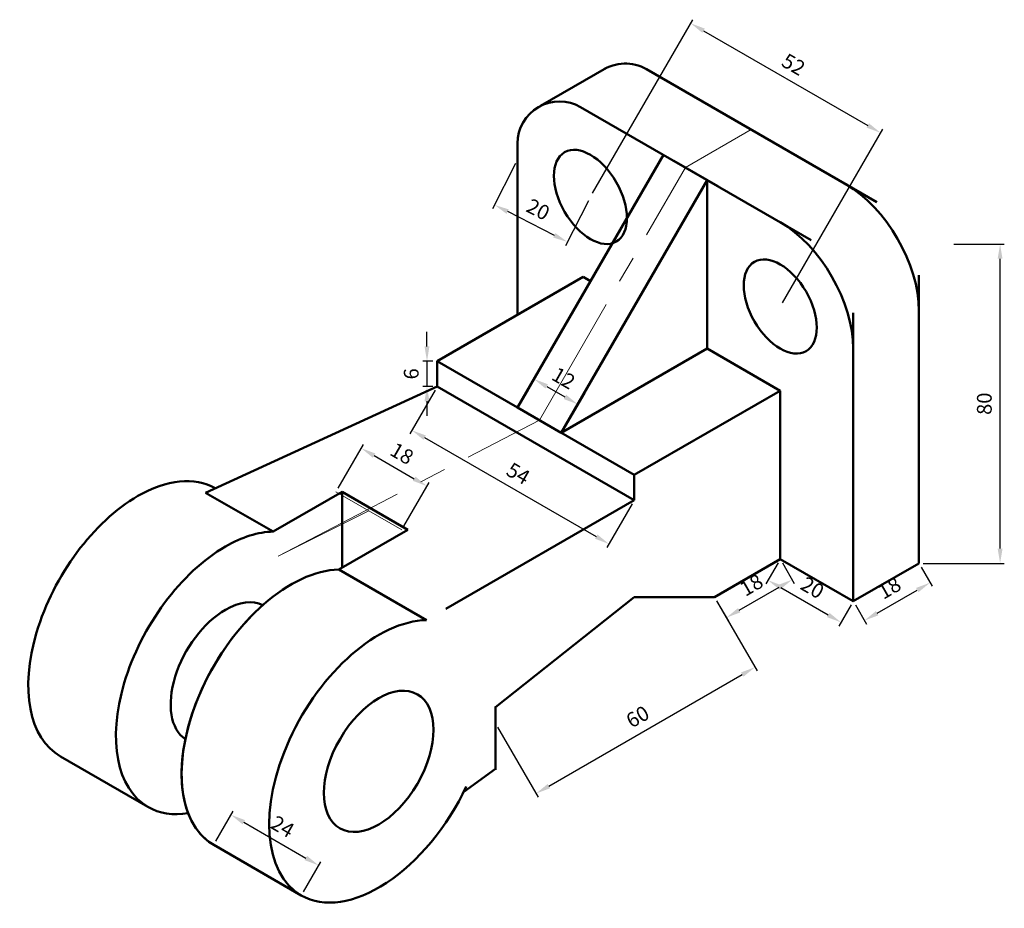
# Model space of a CAD drawing. Units: millimetres. Extents: x 4002 to 4236, y 1032 to 1243.
import ezdxf

# ---------------------------------------------------------------- set-up
doc = ezdxf.new("R2010")
doc.units = ezdxf.units.MM
doc.linetypes.add('CENTER', pattern=[50.8, 31.75, -6.35, 6.35, -6.35])
for name, color, linetype, lineweight in [('M-CNTR', 1, 'CENTER', 18), ('M-DIMS', 3, 'Continuous', 25), ('M-OUTL', 7, 'Continuous', 50)]:
    doc.layers.add(name, color=color, linetype=linetype, lineweight=lineweight)
doc.styles.get("Standard").update_dxf_attribs({"font": 'arial.ttf'})
doc.dimstyles.new('AM_ISO$0', dxfattribs={"dimtxt": 3.5, "dimasz": 3.5, "dimexe": 1, "dimexo": 1, "dimgap": 1.5, "dimtad": 1, "dimdsep": 46, "dimtxsty": 'Standard', "dimcen": 0, "dimclrd": 256, "dimclre": 256, "dimclrt": 2, "dimadec": 0, "dimazin": 2, "dimtp": 0.1, "dimtm": 0.1, "dimtfac": 0.71, "dimtdec": 3, "dimtmove": 0, "dimatfit": 3, "dimfxl": 1, "dimlwd": -1, "dimlwe": -1, "dimarcsym": 1})

# ---------------------------------------------------------------- blocks, each defined once
blk = doc.blocks.new('*D3')
at = {"layer": 'Defpoints', "color": 0, "transparency": 16777216}
for p in [(4206.53, 1216.44), (4137.7, 1201.21), (4182.73, 1175.21)]:
    blk.add_point(p, dxfattribs=at)
at = {"layer": 'M-DIMS', "color": 0, "linetype": 'ByBlock', "transparency": 16777216}
for p, q in [((4138.2, 1202.08), (4162, 1243.3)), ((4164.53, 1240.69), (4203.5, 1218.19)), ((4183.23, 1176.08), (4207.03, 1217.3))]:
    blk.add_line(p, q, dxfattribs=at)
at = {"layer": 'M-DIMS', "color": 0, "transparency": 16777216}
for points in [[(4164.82, 1241.19), (4164.24, 1240.18), (4161.5, 1242.44)], [(4203.79, 1218.69), (4203.21, 1217.68), (4206.53, 1216.44)]]:
    blk.add_solid(points, dxfattribs=at)
at = {"layer": 'M-DIMS', "color": 0, "transparency": 16777216, "insert": (4185.66, 1232.28), "char_height": 3.5, "attachment_point": 5, "rotation": 330}
blk.add_mtext('52', dxfattribs=at)
blk = doc.blocks.new('*D4')
at = {"layer": 'Defpoints', "color": 0, "transparency": 16777216}
for p in [(4167.14, 1106.21), (4176.75, 1089.57), (4115.18, 1076.21)]:
    blk.add_point(p, dxfattribs=at)
at = {"layer": 'M-DIMS', "color": 0, "linetype": 'ByBlock', "transparency": 16777216}
for p, q in [((4167.64, 1105.35), (4177.25, 1088.71)), ((4127.82, 1061.32), (4173.72, 1087.82)), ((4115.68, 1075.35), (4125.29, 1058.71))]:
    blk.add_line(p, q, dxfattribs=at)
at = {"layer": 'M-DIMS', "color": 0, "transparency": 16777216}
for points in [[(4173.43, 1088.33), (4174.01, 1087.32), (4176.75, 1089.57)], [(4127.53, 1061.83), (4128.11, 1060.82), (4124.79, 1059.57)]]:
    blk.add_solid(points, dxfattribs=at)
at = {"layer": 'M-DIMS', "color": 0, "transparency": 16777216, "insert": (4149.12, 1077.42), "char_height": 3.5, "attachment_point": 5, "rotation": 30}
blk.add_mtext('60', dxfattribs=at)
blk = doc.blocks.new('*D5')
at = {"layer": 'Defpoints', "color": 0, "transparency": 16777216}
for p in [(4182.73, 1115.21), (4200.05, 1105.21), (4197.16, 1100.21)]:
    blk.add_point(p, dxfattribs=at)
at = {"layer": 'M-DIMS', "color": 0, "linetype": 'ByBlock', "transparency": 16777216}
for p, q in [((4182.23, 1114.35), (4179.34, 1109.34)), ((4182.87, 1108.46), (4194.13, 1101.96)), ((4199.55, 1104.35), (4196.66, 1099.34))]:
    blk.add_line(p, q, dxfattribs=at)
at = {"layer": 'M-DIMS', "color": 0, "transparency": 16777216}
for points in [[(4183.16, 1108.96), (4182.58, 1107.95), (4179.84, 1110.21)], [(4194.42, 1102.46), (4193.84, 1101.45), (4197.16, 1100.21)]]:
    blk.add_solid(points, dxfattribs=at)
at = {"layer": 'M-DIMS', "color": 0, "transparency": 16777216, "insert": (4190.15, 1108.06), "char_height": 3.5, "attachment_point": 5, "rotation": 330}
blk.add_mtext('20', dxfattribs=at)
blk = doc.blocks.new('*D6')
at = {"layer": 'Defpoints', "color": 0, "transparency": 16777216}
for p in [(4182.73, 1115.21), (4185.54, 1110.34), (4167.14, 1106.21)]:
    blk.add_point(p, dxfattribs=at)
at = {"layer": 'M-DIMS', "color": 0, "linetype": 'ByBlock', "transparency": 16777216}
for p, q in [((4183.23, 1114.35), (4186.04, 1109.47)), ((4172.99, 1103.09), (4182.51, 1108.59)), ((4167.64, 1105.35), (4170.46, 1100.47))]:
    blk.add_line(p, q, dxfattribs=at)
at = {"layer": 'M-DIMS', "color": 0, "transparency": 16777216}
for points in [[(4182.22, 1109.09), (4182.81, 1108.08), (4185.54, 1110.34)], [(4172.7, 1103.59), (4173.28, 1102.58), (4169.96, 1101.34)]]:
    blk.add_solid(points, dxfattribs=at)
at = {"layer": 'M-DIMS', "color": 0, "transparency": 16777216, "insert": (4176.11, 1108.69), "char_height": 3.5, "attachment_point": 5, "rotation": 30}
blk.add_mtext('18', dxfattribs=at)
blk = doc.blocks.new('*D7')
at = {"layer": 'Defpoints', "color": 0, "transparency": 16777216}
for p in [(4215.64, 1114.21), (4218.28, 1109.64), (4200.05, 1105.21)]:
    blk.add_point(p, dxfattribs=at)
at = {"layer": 'M-DIMS', "color": 0, "linetype": 'ByBlock', "transparency": 16777216}
for p, q in [((4216.14, 1113.35), (4218.78, 1108.77)), ((4205.72, 1102.39), (4215.25, 1107.89)), ((4200.55, 1104.35), (4203.19, 1099.77))]:
    blk.add_line(p, q, dxfattribs=at)
at = {"layer": 'M-DIMS', "color": 0, "transparency": 16777216}
for points in [[(4214.96, 1108.39), (4215.54, 1107.38), (4218.28, 1109.64)], [(4205.43, 1102.89), (4206.01, 1101.88), (4202.69, 1100.64)]]:
    blk.add_solid(points, dxfattribs=at)
at = {"layer": 'M-DIMS', "color": 0, "transparency": 16777216, "insert": (4208.84, 1107.98), "char_height": 3.5, "attachment_point": 5, "rotation": 30}
blk.add_mtext('18', dxfattribs=at)
blk = doc.blocks.new('*D8')
at = {"layer": 'Defpoints', "color": 0, "transparency": 16777216}
for p in [(4222.89, 1190.03), (4234.89, 1190.03), (4215.64, 1114.21)]:
    blk.add_point(p, dxfattribs=at)
at = {"layer": 'M-DIMS', "color": 0, "linetype": 'ByBlock', "transparency": 16777216}
for p, q in [((4223.89, 1190.03), (4235.89, 1190.03)), ((4234.89, 1117.71), (4234.89, 1186.53)), ((4216.64, 1114.21), (4235.89, 1114.21))]:
    blk.add_line(p, q, dxfattribs=at)
at = {"layer": 'M-DIMS', "color": 0, "transparency": 16777216}
for points in [[(4234.31, 1186.53), (4235.47, 1186.53), (4234.89, 1190.03)], [(4234.31, 1117.71), (4235.47, 1117.71), (4234.89, 1114.21)]]:
    blk.add_solid(points, dxfattribs=at)
at = {"layer": 'M-DIMS', "color": 0, "transparency": 16777216, "insert": (4231.6, 1152.12), "char_height": 3.5, "attachment_point": 5, "rotation": 90}
blk.add_mtext('80', dxfattribs=at)
blk = doc.blocks.new('*D9')
at = {"layer": 'Defpoints', "color": 0, "transparency": 16777216}
for p in [(4101.32, 1156.21), (4148.09, 1129.21), (4142.09, 1118.82)]:
    blk.add_point(p, dxfattribs=at)
at = {"layer": 'M-DIMS', "color": 0, "linetype": 'ByBlock', "transparency": 16777216}
for p, q in [((4100.82, 1155.35), (4094.82, 1144.95)), ((4098.36, 1144.07), (4139.06, 1120.57)), ((4147.59, 1128.35), (4141.59, 1117.95))]:
    blk.add_line(p, q, dxfattribs=at)
at = {"layer": 'M-DIMS', "color": 0, "transparency": 16777216}
for points in [[(4098.65, 1144.58), (4098.06, 1143.57), (4095.32, 1145.82)], [(4139.35, 1121.08), (4138.77, 1120.07), (4142.09, 1118.82)]]:
    blk.add_solid(points, dxfattribs=at)
at = {"layer": 'M-DIMS', "color": 0, "transparency": 16777216, "insert": (4120.35, 1135.16), "char_height": 3.5, "attachment_point": 5, "rotation": 330}
blk.add_mtext('54', dxfattribs=at)
blk = doc.blocks.new('*D10')
at = {"layer": 'Defpoints', "color": 0, "transparency": 16777216}
for p in [(4101.32, 1162.21), (4098.92, 1156.21), (4101.32, 1156.21)]:
    blk.add_point(p, dxfattribs=at)
at = {"layer": 'M-DIMS', "color": 0, "linetype": 'ByBlock', "transparency": 16777216}
for p, q in [((4098.92, 1165.71), (4098.92, 1169.21)), ((4100.32, 1162.21), (4097.92, 1162.21)), ((4098.92, 1162.21), (4098.92, 1156.21)), ((4100.32, 1156.21), (4097.92, 1156.21)), ((4098.92, 1152.71), (4098.92, 1149.21))]:
    blk.add_line(p, q, dxfattribs=at)
at = {"layer": 'M-DIMS', "color": 0, "transparency": 16777216}
for points in [[(4098.33, 1165.71), (4099.5, 1165.71), (4098.92, 1162.21)], [(4098.33, 1152.71), (4099.5, 1152.71), (4098.92, 1156.21)]]:
    blk.add_solid(points, dxfattribs=at)
at = {"layer": 'M-DIMS', "color": 0, "transparency": 16777216, "insert": (4095.63, 1159.21), "char_height": 3.5, "attachment_point": 5, "rotation": 90}
blk.add_mtext('6', dxfattribs=at)
blk = doc.blocks.new('*D11')
at = {"layer": 'Defpoints', "color": 0, "transparency": 16777216}
for p in [(4134.68, 1151.99), (4120.38, 1151.22), (4130.77, 1145.22)]:
    blk.add_point(p, dxfattribs=at)
at = {"layer": 'M-DIMS', "color": 0, "linetype": 'ByBlock', "transparency": 16777216}
for p, q in [((4120.88, 1152.08), (4124.79, 1158.86)), ((4127.32, 1156.24), (4131.65, 1153.74)), ((4131.27, 1146.08), (4135.18, 1152.86))]:
    blk.add_line(p, q, dxfattribs=at)
at = {"layer": 'M-DIMS', "color": 0, "transparency": 16777216}
for points in [[(4127.61, 1156.74), (4127.03, 1155.73), (4124.29, 1157.99)], [(4131.94, 1154.24), (4131.36, 1153.23), (4134.68, 1151.99)]]:
    blk.add_solid(points, dxfattribs=at)
at = {"layer": 'M-DIMS', "color": 0, "transparency": 16777216, "insert": (4131.11, 1157.81), "char_height": 3.5, "attachment_point": 5, "rotation": 330}
blk.add_mtext('12', dxfattribs=at)
blk = doc.blocks.new('*D12')
at = {"layer": 'Defpoints', "color": 0, "transparency": 16777216}
for p in [(4120.38, 1210.02), (4137.7, 1201.21), (4114.94, 1199.32)]:
    blk.add_point(p, dxfattribs=at)
at = {"layer": 'M-DIMS', "color": 0, "linetype": 'ByBlock', "transparency": 16777216}
for p, q in [((4119.92, 1209.13), (4114.49, 1198.43)), ((4137.24, 1200.32), (4131.81, 1189.62)), ((4129.14, 1192.1), (4118.06, 1197.74))]:
    blk.add_line(p, q, dxfattribs=at)
at = {"layer": 'M-DIMS', "color": 0, "transparency": 16777216}
for points in [[(4118.32, 1198.26), (4117.79, 1197.22), (4114.94, 1199.32)], [(4129.4, 1192.62), (4128.87, 1191.58), (4132.26, 1190.52)]]:
    blk.add_solid(points, dxfattribs=at)
at = {"layer": 'M-DIMS', "color": 0, "transparency": 16777216, "insert": (4125.09, 1197.85), "char_height": 3.5, "attachment_point": 5, "rotation": 333.0509}
blk.add_mtext('20', dxfattribs=at)
blk = doc.blocks.new('*D13')
at = {"layer": 'Defpoints', "color": 0, "transparency": 16777216}
for p in [(4077.33, 1131.17), (4098.91, 1132.56), (4092.91, 1122.17)]:
    blk.add_point(p, dxfattribs=at)
at = {"layer": 'M-DIMS', "color": 0, "linetype": 'ByBlock', "transparency": 16777216}
for p, q in [((4077.83, 1132.04), (4083.83, 1142.43)), ((4086.36, 1139.81), (4095.88, 1134.31)), ((4093.41, 1123.04), (4099.41, 1133.43))]:
    blk.add_line(p, q, dxfattribs=at)
at = {"layer": 'M-DIMS', "color": 0, "transparency": 16777216}
for points in [[(4086.65, 1140.32), (4086.06, 1139.31), (4083.33, 1141.56)], [(4096.17, 1134.82), (4095.59, 1133.81), (4098.91, 1132.56)]]:
    blk.add_solid(points, dxfattribs=at)
at = {"layer": 'M-DIMS', "color": 0, "transparency": 16777216, "insert": (4092.76, 1139.91), "char_height": 3.5, "attachment_point": 5, "rotation": 330}
blk.add_mtext('18', dxfattribs=at)
blk = doc.blocks.new('*D14')
at = {"layer": 'Defpoints', "color": 0, "transparency": 16777216}
for p in [(4048.31, 1047.39), (4073.21, 1042.51), (4069.1, 1035.39)]:
    blk.add_point(p, dxfattribs=at)
at = {"layer": 'M-DIMS', "color": 0, "linetype": 'ByBlock', "transparency": 16777216}
for p, q in [((4048.81, 1048.26), (4052.92, 1055.38)), ((4055.45, 1052.76), (4070.18, 1044.26)), ((4069.6, 1036.26), (4073.71, 1043.38))]:
    blk.add_line(p, q, dxfattribs=at)
at = {"layer": 'M-DIMS', "color": 0, "transparency": 16777216}
for points in [[(4055.75, 1053.27), (4055.16, 1052.26), (4052.42, 1054.51)], [(4070.47, 1044.77), (4069.88, 1043.76), (4073.21, 1042.51)]]:
    blk.add_solid(points, dxfattribs=at)
at = {"layer": 'M-DIMS', "color": 0, "transparency": 16777216, "insert": (4064.44, 1051.33), "char_height": 3.5, "attachment_point": 5, "rotation": 330}
blk.add_mtext('24', dxfattribs=at)

msp = doc.modelspace()

# ---------------------------------------------------------------- linework, layer by layer
at = {"layer": 'M-CNTR'}
for p, q in [((4160.214, 1208.213), (4175.802, 1217.213)), ((4125.573, 1148.213), (4160.214, 1208.213)), ((4063.646, 1115.952), (4125.573, 1148.213)), ((4092.914, 1122.17), (4077.325, 1131.17)), ((4063.646, 1115.952), (4085.12, 1126.67)), ((4085.12, 1126.67), (4092.914, 1122.17))]:
    msp.add_line(p, q, dxfattribs=at)
at = {"layer": 'M-OUTL'}
for p, q in [((4141.482, 1231.831), (4125.864, 1222.816)), ((4205.64, 1199.986), (4150.965, 1231.552)), ((4125.864, 1222.816), (4125.377, 1222.552)), ((4125.817, 1222.792), (4125.377, 1222.552)), ((4135.377, 1222.552), (4190.051, 1190.986)), ((4120.377, 1173.213), (4120.377, 1213.892)), ((4155.019, 1211.217), (4120.378, 1151.217)), ((4167.91, 1203.769), (4157.518, 1209.769)), ((4162.714, 1206.769), (4167.91, 1203.769)), ((4165.409, 1205.213), (4130.768, 1145.213)), ((4165.409, 1205.213), (4165.409, 1165.213)), ((4101.324, 1162.213), (4135.965, 1182.213)), ((4137.697, 1181.213), (4135.965, 1182.213)), ((4215.64, 1114.213), (4215.64, 1182.666)), ((4200.051, 1173.666), (4200.051, 1105.213)), ((4165.409, 1165.213), (4130.768, 1145.213)), ((4182.731, 1155.213), (4165.41, 1165.213)), ((4120.377, 1151.213), (4101.324, 1162.213)), ((4101.324, 1162.213), (4101.324, 1156.213)), ((4101.324, 1156.213), (4046.393, 1131.004)), ((4148.09, 1129.213), (4101.324, 1156.213)), ((4125.573, 1148.213), (4115.181, 1154.213)), ((4120.378, 1151.217), (4122.816, 1155.437)), ((4130.768, 1145.213), (4136.261, 1154.727)), ((4182.731, 1155.213), (4148.09, 1135.213)), ((4182.731, 1115.213), (4182.731, 1155.213)), ((4120.377, 1151.213), (4125.573, 1148.213)), ((4148.09, 1135.213), (4120.377, 1151.213)), ((4130.768, 1145.213), (4120.378, 1151.217)), ((4148.09, 1135.213), (4148.09, 1129.213)), ((4062.42, 1121.751), (4046.393, 1131.004)), ((4078.808, 1131.213), (4062.42, 1121.751)), ((4094.396, 1122.213), (4078.808, 1131.213)), ((4078.808, 1113.213), (4078.808, 1131.213)), ((4148.09, 1129.213), (4103.424, 1103.425)), ((4094.396, 1122.213), (4078.008, 1112.751)), ((4182.731, 1115.213), (4167.142, 1106.213)), ((4200.051, 1105.213), (4182.731, 1115.213)), ((4200.051, 1105.213), (4182.731, 1115.213)), ((4098.793, 1100.751), (4078.008, 1112.751)), ((4200.051, 1105.213), (4215.64, 1114.213)), ((4148.09, 1106.213), (4115.181, 1080.099)), ((4167.142, 1106.213), (4148.09, 1106.213)), ((4115.181, 1065.213), (4115.181, 1080.213)), ((4115.181, 1076.213), (4115.181, 1065.43)), ((4032.724, 1056.393), (4011.939, 1068.393)), ((4115.181, 1065.43), (4107.643, 1059.96)), ((4048.312, 1047.393), (4069.097, 1035.393))]:
    msp.add_line(p, q, dxfattribs=at)
for centre, end in [((4145.965, 1222.892), 123.35242), ((4130.377, 1213.892), 180)]:
    msp.add_arc(centre, 10, 60, end, dxfattribs=at)
for centre, major_axis in [((4137.697, 1201.213), (6.124, -10.607)), ((4182.731, 1175.213), (6.124, -10.607)), ((4087.468, 1067.213), (-9.186, -15.91))]:
    msp.add_ellipse(centre, major_axis=major_axis, ratio=0.5773503, dxfattribs=at)
for centre, major_axis, start_param, end_param in [((4198.319, 1184.213), (-12.247, 21.213), 3.9269908, 5.4977871), ((4182.731, 1175.213), (-12.247, 21.213), 3.9269908, 5.4977871), ((4030.31, 1100.213), (18.371, 31.82), 0.0011217, 0.7853982), ((4030.31, 1100.213), (18.371, 31.82), 0.7853982, 3.1415927), ((4051.095, 1088.213), (18.371, 31.82), 0.3343714, 0.7853982), ((4051.095, 1088.213), (18.371, 31.82), 0.7853982, 3.1415927), ((4066.683, 1079.213), (-18.371, -31.82), 3.475964, 6.2831853), ((4051.095, 1088.213), (9.186, 15.91), 0.0353627, 0.7853982), ((4051.095, 1088.213), (9.186, 15.91), 0.7853982, 3.1062299), ((4066.683, 1079.213), (-18.371, -31.82), 4.3111294, 6.2831853), ((4087.468, 1067.213), (-18.371, -31.82), 3.475964, 6.2831853), ((4087.468, 1067.213), (-18.371, -31.82), 0, 1.7126934), ((4051.095, 1088.213), (18.371, 31.82), 3.1415927, 3.5797417)]:
    msp.add_ellipse(centre, major_axis=major_axis, ratio=0.5773503, start_param=start_param, end_param=end_param, dxfattribs=at)

# ---------------------------------------------------------------- dimensions: what is measured, and where the dimension line sits
at = {"layer": 'M-DIMS'}
for p1, p2, distance, override, picture, middle in [((4137.697, 1201.213), (4182.731, 1175.213), 47.602, {"dimpost": '', "dimclrd": 0, "dimclre": 0, "dimclrt": 0}, '*D3', (4185.659, 1232.284)), ((4101.324, 1162.213), (4101.324, 1156.213), -2.406, {"dimclrd": 0, "dimclre": 0, "dimclrt": 0}, '*D10', (4095.631, 1159.213)), ((4120.378, 1151.217), (4130.771, 1145.217), 7.821, {"dimclrd": 0, "dimclre": 0, "dimclrt": 0}, '*D11', (4131.113, 1157.81)), ((4101.324, 1156.213), (4148.09, 1129.213), -12, {"dimpost": '', "dimclrd": 0, "dimclre": 0, "dimclrt": 0}, '*D9', (4120.347, 1135.161)), ((4077.325, 1131.17), (4092.914, 1122.17), 12, {"dimclrd": 0, "dimclre": 0, "dimclrt": 0}, '*D13', (4092.763, 1139.909)), ((4167.142, 1106.213), (4182.731, 1115.213), -5.628, {"dimclrd": 0, "dimclre": 0, "dimclrt": 0}, '*D6', (4176.107, 1108.685)), ((4182.731, 1115.213), (4200.051, 1105.213), -5.777, {"dimclrd": 0, "dimclre": 0, "dimclrt": 0}, '*D5', (4190.146, 1108.056)), ((4200.051, 1105.213), (4215.64, 1114.213), -5.282, {"dimclrd": 0, "dimclre": 0, "dimclrt": 0}, '*D7', (4208.843, 1107.985)), ((4115.181, 1076.213), (4167.142, 1106.213), -19.212, {"dimclrd": 0, "dimclre": 0, "dimclrt": 0}, '*D4', (4149.124, 1077.421)), ((4048.312, 1047.393), (4069.097, 1035.393), 8.222, {"dimclrd": 0, "dimclre": 0, "dimclrt": 0}, '*D14', (4064.444, 1051.334))]:
    dim = msp.add_aligned_dim(p1=p1, p2=p2, distance=distance, dimstyle='AM_ISO$0', override=override, dxfattribs=at)
    dim.commit()
    dim.dimension.update_dxf_attribs({"geometry": picture, "text_midpoint": middle})
dim = msp.add_aligned_dim(p1=(4137.697, 1201.213), p2=(4120.377, 1210.018), distance=12, text='20', dimstyle='AM_ISO$0', override={"dimpost": '', "dimclrd": 0, "dimclre": 0, "dimclrt": 0}, dxfattribs=at)
dim.commit()
dim.dimension.update_dxf_attribs({"geometry": '*D12', "text_midpoint": (4125.088, 1197.849)})
dim = msp.add_linear_dim(base=(4234.889, 1190.027), p1=(4215.64, 1114.213), p2=(4222.889, 1190.027), angle=90, text='80', dimstyle='AM_ISO$0', override={"dimpost": '', "dimclrd": 0, "dimclre": 0, "dimclrt": 0}, dxfattribs=at)
dim.commit()
dim.dimension.update_dxf_attribs({"geometry": '*D8', "text_midpoint": (4231.602, 1152.12)})

doc.saveas('drawing.dxf')
